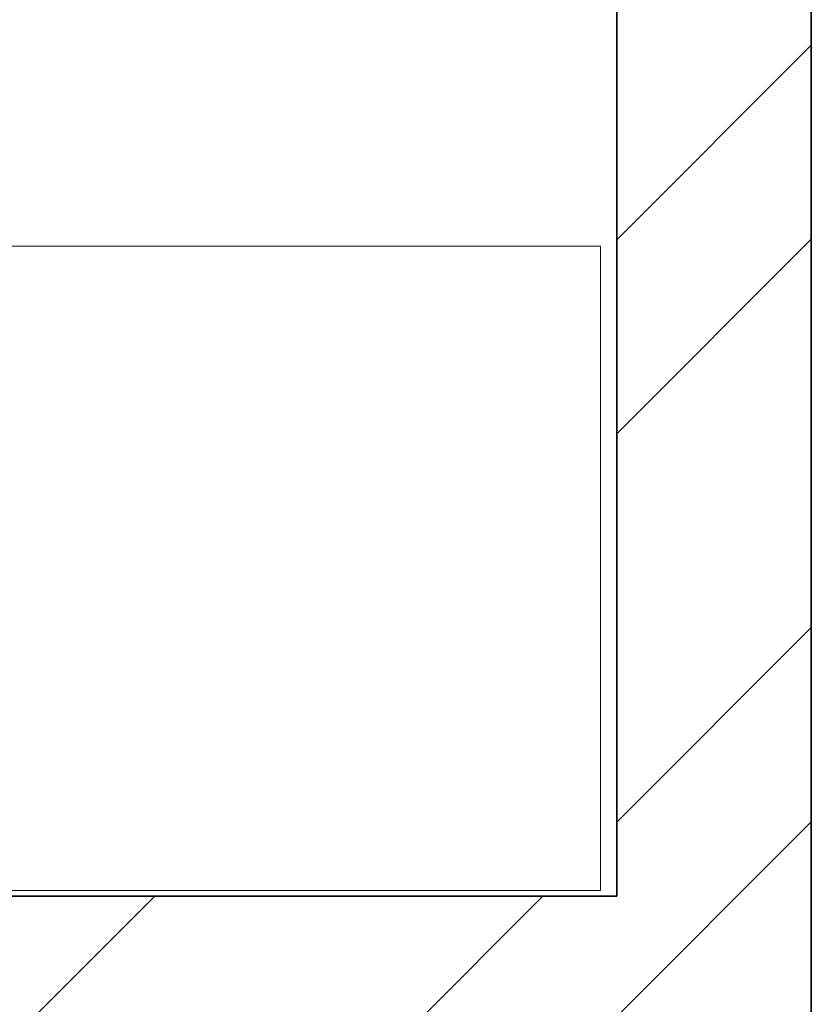
# Model space of a CAD drawing. Units: inches. Extents: x 2168 to 3056, y 1130 to 2629.
# Tile 40 of 42: x 2846 to 2864, y 2263 to 2286. Entities that reach past the tile are written whole.
import ezdxf

# ---------------------------------------------------------------- set-up
doc = ezdxf.new("R2010")
doc.units = ezdxf.units.IN
doc.layers.add('A-FLOR-CASE', color=71, linetype='Continuous', lineweight=18)
doc.layers.add('A-WALL', color=7, linetype='Continuous', lineweight=35)
doc.layers.add('A-WALL-PATT', color=143, linetype='Continuous', lineweight=13, true_color=0x7aafdf)

# ---------------------------------------------------------------- blocks, each defined once
blk = doc.blocks.new('CUPBOARD-BEDROOM')
blk.add_lwpolyline([(0, 14.894), (70.359, 14.894), (70.359, 0), (0, 0)], close=True)

msp = doc.modelspace()

# ---------------------------------------------------------------- hatches: boundary and pattern name
at = {"layer": 'A-WALL-PATT'}
h = msp.add_hatch(dxfattribs=at)
h.set_pattern_fill('ANSI32', color=256)
h.paths.add_polyline_path([(2463.796, 2409.389), (2467.387, 2409.389), (2467.387, 2413.889), (2454.768, 2413.889), (2454.768, 2411.639), (2454.768, 2409.389), (2459.296, 2409.389), (2459.296, 2265.389), (2455.644, 2265.389), (2455.644, 2260.889), (2467.349, 2260.889), (2467.349, 2263.139), (2467.349, 2265.389), (2463.796, 2265.389)])
h.paths.add_polyline_path([(2431.596, 2413.889), (2409.647, 2413.889), (2409.647, 2409.389), (2431.596, 2409.389), (2431.596, 2411.639)])
h.paths.add_polyline_path([(2349.647, 2413.889), (2331.796, 2413.889), (2331.796, 2362.671), (2336.296, 2362.671), (2336.296, 2409.389), (2349.647, 2409.389), (2349.647, 2411.639)])
h.paths.add_polyline_path([(2634.149, 2411.639), (2634.149, 2413.889), (2562.293, 2413.889), (2562.293, 2409.389), (2595.796, 2409.389), (2595.796, 2280.309), (2595.826, 2280.309), (2595.826, 2265.389), (2499.91, 2265.389), (2499.91, 2260.889), (2550.796, 2260.889), (2550.796, 2117.308), (2555.296, 2117.308), (2555.296, 2168.08), (2571.93, 2168.08), (2571.93, 2176.889), (2559.796, 2176.889), (2559.796, 2256.389), (2640.796, 2256.389), (2640.796, 2176.889), (2626.428, 2176.889), (2626.428, 2168.08), (2645.296, 2168.08), (2645.296, 2116.637), (2649.796, 2116.637), (2649.796, 2260.889), (2691.251, 2260.889), (2691.251, 2263.139), (2691.251, 2265.389), (2670.655, 2265.389), (2670.655, 2265.365), (2600.296, 2265.365), (2600.296, 2280.258), (2600.296, 2409.389), (2634.149, 2409.389)])
h.paths.add_polyline_path([(2600.296, 2473.889), (2612.84, 2473.889), (2612.84, 2478.389), (2572.636, 2478.389), (2572.636, 2473.889), (2595.796, 2473.889), (2595.796, 2413.889), (2600.296, 2413.889)])
h.paths.add_polyline_path([(2535.796, 2473.889), (2548.636, 2473.889), (2548.636, 2478.389), (2531.396, 2478.389), (2531.396, 2413.889), (2521.6, 2413.889), (2521.6, 2409.389), (2539.239, 2409.389), (2539.239, 2411.639), (2539.239, 2413.889), (2535.796, 2413.889)])
h.paths.add_polyline_path([(2664.796, 2478.389), (2636.84, 2478.389), (2636.84, 2473.889), (2660.296, 2473.889), (2660.296, 2413.889), (2656.165, 2413.889), (2656.165, 2409.389), (2671.684, 2409.389), (2671.684, 2411.639), (2671.684, 2413.889), (2664.796, 2413.889)])
h.paths.add_polyline_path([(2705.942, 2413.889), (2695.684, 2413.889), (2695.684, 2409.389), (2705.942, 2409.389)])
h.paths.add_polyline_path([(2741.35, 2413.889), (2728.733, 2413.889), (2728.733, 2411.639), (2728.733, 2409.389), (2732.296, 2409.389), (2732.296, 2265.389), (2725.733, 2265.389), (2725.733, 2260.889), (2740.917, 2260.889), (2740.917, 2263.139), (2740.917, 2265.389), (2736.796, 2265.389), (2736.796, 2409.389), (2741.35, 2409.389)])
h.paths.add_polyline_path([(2785.655, 2413.889), (2764.546, 2413.889), (2764.486, 2409.389), (2785.655, 2409.389), (2785.655, 2411.639)])
h.paths.add_polyline_path([(2864.296, 2413.889), (2845.655, 2413.889), (2845.655, 2409.389), (2859.796, 2409.389), (2859.796, 2368.425), (2864.296, 2368.425)])
h.paths.add_polyline_path([(2864.296, 2308.425), (2862.046, 2308.425), (2859.796, 2308.425), (2859.796, 2265.389), (2774.483, 2265.389), (2774.483, 2263.139), (2774.483, 2260.889), (2781.796, 2260.889), (2781.796, 2226.654), (2786.296, 2226.654), (2786.296, 2260.889), (2859.796, 2260.889), (2859.796, 2241.352), (2864.296, 2241.352)])
h.paths.add_polyline_path([(2864.296, 2217.352), (2862.046, 2217.352), (2859.796, 2217.352), (2859.796, 2200.889), (2786.296, 2200.889), (2786.296, 2205.931), (2784.046, 2205.931), (2781.796, 2205.931), (2781.796, 2150.974), (2786.296, 2150.974), (2786.296, 2161.889), (2859.796, 2161.889), (2859.796, 2144.419), (2864.296, 2144.419)])
h.paths.add_polyline_path([(2859.796, 2196.389), (2859.796, 2166.389), (2786.296, 2166.389), (2786.296, 2196.389)], flags=16)
h.paths.add_polyline_path([(2864.296, 2108.419), (2862.046, 2108.419), (2859.796, 2108.419), (2859.796, 2080.889), (2786.296, 2080.889), (2786.296, 2111.993), (2781.796, 2111.993), (2781.796, 2080.889), (2649.796, 2080.889), (2649.796, 2086.036), (2647.546, 2086.036), (2645.296, 2086.036), (2645.296, 2071.739), (2649.796, 2071.739), (2649.796, 2076.389), (2781.796, 2076.389), (2781.796, 2041.792), (2786.296, 2041.792), (2786.296, 2076.389), (2859.796, 2076.389), (2859.796, 2058.577), (2864.296, 2058.577)])
h.paths.add_polyline_path([(2864.296, 2022.577), (2859.796, 2022.577), (2859.796, 1992.389), (2786.296, 1992.389), (2786.296, 1999.573), (2781.796, 1999.573), (2781.796, 1848.085), (2784.046, 1848.085), (2786.296, 1848.085), (2786.296, 1851.389), (2859.796, 1851.389), (2859.796, 1838.258), (2864.296, 1838.258)], flags=17)
h.paths.add_polyline_path([(2859.796, 1987.889), (2859.796, 1855.889), (2786.296, 1855.889), (2786.296, 1987.889)], flags=16)
h.paths.add_polyline_path([(2823.046, 1987.889), (2841.421, 1921.889), (2823.046, 1855.889)], flags=0)
h.paths.add_polyline_path([(2864.296, 1814.258), (2859.796, 1814.258), (2859.796, 1791.389), (2786.296, 1791.389), (2786.296, 1825.658), (2784.046, 1825.658), (2781.796, 1825.658), (2781.796, 1791.389), (2720.155, 1791.389), (2720.155, 1791.265), (2649.796, 1791.265), (2649.796, 1806.159), (2649.796, 2038.983), (2647.546, 2038.983), (2645.296, 2038.983), (2645.296, 1783.925), (2649.796, 1783.925), (2649.796, 1786.889), (2781.796, 1786.889), (2781.796, 1746.789), (2786.296, 1746.789), (2786.296, 1786.889), (2859.796, 1786.889), (2859.796, 1770.083), (2864.296, 1770.083)])
h.paths.add_polyline_path([(2864.296, 1734.083), (2862.046, 1734.083), (2859.796, 1734.083), (2859.796, 1705.889), (2786.296, 1705.889), (2786.296, 1714.166), (2781.796, 1714.166), (2781.796, 1660.527), (2786.296, 1660.527), (2786.296, 1666.889), (2859.796, 1666.889), (2859.796, 1648.342), (2864.296, 1648.342)])
h.paths.add_polyline_path([(2786.296, 1701.389), (2859.796, 1701.389), (2859.796, 1671.389), (2786.296, 1671.389)], flags=16)
h.paths.add_polyline_path([(2649.796, 1756.576), (2647.546, 1756.576), (2645.296, 1756.576), (2645.296, 1606.889), (2555.296, 1606.889), (2555.296, 1749.513), (2553.046, 1749.513), (2550.796, 1749.513), (2550.796, 1606.889), (2503.006, 1606.889), (2503.006, 1604.639), (2503.006, 1602.389), (2595.796, 1602.389), (2595.849, 1602.389), (2595.849, 1587.495), (2595.796, 1458.389), (2561.502, 1458.389), (2561.502, 1456.139), (2561.502, 1453.889), (2595.796, 1453.889), (2595.796, 1381.889), (2573.438, 1381.889), (2573.438, 1377.389), (2613.01, 1377.389), (2613.01, 1379.639), (2613.01, 1381.889), (2600.296, 1381.889), (2600.296, 1453.889), (2634.327, 1453.889), (2634.327, 1458.389), (2600.296, 1458.389), (2600.296, 1602.389), (2670.655, 1602.389), (2694.095, 1602.389), (2694.095, 1606.889), (2649.796, 1606.889)])
h.paths.add_polyline_path([(2736.796, 1602.389), (2741.562, 1602.389), (2741.562, 1606.889), (2726.203, 1606.889), (2726.203, 1604.639), (2726.203, 1602.389), (2732.296, 1602.389), (2732.296, 1458.389), (2727.899, 1458.389), (2727.899, 1453.889), (2740.821, 1453.889), (2740.821, 1456.139), (2740.821, 1458.389), (2736.796, 1458.389)])
h.paths.add_polyline_path([(2859.796, 1606.889), (2786.296, 1606.889), (2786.296, 1637.334), (2784.046, 1637.334), (2781.796, 1637.334), (2781.796, 1606.889), (2775.612, 1606.889), (2775.612, 1602.389), (2859.796, 1602.389)])
h.paths.add_polyline_path([(2864.296, 1624.342), (2862.046, 1624.342), (2859.796, 1624.342), (2859.796, 1570.39), (2864.296, 1570.39)])
h.paths.add_polyline_path([(2864.296, 1510.39), (2862.046, 1510.39), (2859.796, 1510.39), (2859.796, 1458.389), (2846.735, 1458.389), (2846.735, 1456.139), (2846.735, 1453.889), (2864.296, 1453.889)])
h.paths.add_polyline_path([(2786.735, 1458.389), (2765.444, 1458.389), (2765.444, 1453.889), (2786.735, 1453.889)])
h.paths.add_polyline_path([(2706.004, 1458.389), (2695.36, 1458.389), (2695.36, 1453.889), (2706.004, 1453.889), (2706.004, 1456.139)])
h.paths.add_polyline_path([(2671.36, 1456.139), (2671.36, 1458.389), (2655.986, 1458.389), (2655.986, 1456.139), (2655.986, 1453.889), (2660.296, 1453.889), (2660.296, 1381.889), (2637.01, 1381.889), (2637.01, 1377.389), (2664.796, 1377.389), (2664.796, 1453.889), (2671.36, 1453.889)], flags=17)
h.paths.add_polyline_path([(2539.829, 1458.389), (2520.237, 1458.389), (2520.237, 1453.889), (2531.296, 1453.889), (2531.296, 1377.389), (2546.449, 1377.389), (2546.449, 1379.639), (2546.449, 1381.889), (2535.796, 1381.889), (2535.796, 1453.889), (2539.829, 1453.889)], flags=17)
h.paths.add_polyline_path([(2496.237, 1458.389), (2489.13, 1458.389), (2489.13, 1453.889), (2496.237, 1453.889), (2496.237, 1456.139)])
h.paths.add_polyline_path([(2467.433, 1456.139), (2467.433, 1458.389), (2463.796, 1458.389), (2463.796, 1602.389), (2468.242, 1602.389), (2468.242, 1605.7), (2468.242, 1606.889), (2454.602, 1606.889), (2454.602, 1602.389), (2459.296, 1602.389), (2459.296, 1458.389), (2454.24, 1458.389), (2454.24, 1453.889), (2467.433, 1453.889)])
h.paths.add_polyline_path([(2431.601, 1456.139), (2431.601, 1458.389), (2411.386, 1458.389), (2411.386, 1453.889), (2431.601, 1453.889)])
h.paths.add_polyline_path([(2351.386, 1458.389), (2336.296, 1458.389), (2336.296, 1490.693), (2334.046, 1490.693), (2331.796, 1490.693), (2331.796, 1453.889), (2351.386, 1453.889), (2351.386, 1456.139)])
h.paths.add_polyline_path([(2336.296, 1629.705), (2331.796, 1629.705), (2331.796, 1552.317), (2336.296, 1552.317), (2336.296, 1602.389), (2406.655, 1602.389), (2423.472, 1602.389), (2423.472, 1606.889), (2418.796, 1606.889), (2418.796, 1643.678), (2416.546, 1643.678), (2414.296, 1643.678), (2414.296, 1606.889), (2336.296, 1606.889)])
h.paths.add_polyline_path([(2418.796, 1714.384), (2414.296, 1714.384), (2414.296, 1705.889), (2336.296, 1705.889), (2336.296, 1731.324), (2334.046, 1731.324), (2331.796, 1731.324), (2331.796, 1653.705), (2334.046, 1653.705), (2336.296, 1653.705), (2336.296, 1666.889), (2414.296, 1666.889), (2414.296, 1663.589), (2418.796, 1663.589)])
h.paths.add_polyline_path([(2336.296, 1701.389), (2414.296, 1701.389), (2414.296, 1671.389), (2336.296, 1671.389)], flags=16)
h.paths.add_polyline_path([(2555.296, 2040.059), (2550.796, 2040.059), (2550.796, 1791.389), (2550.561, 1791.205), (2480.202, 1791.205), (2418.796, 1791.389), (2418.796, 1825.448), (2416.546, 1825.448), (2414.296, 1825.448), (2414.296, 1791.389), (2336.296, 1791.389), (2336.296, 1806.409), (2331.796, 1806.409), (2331.796, 1767.324), (2336.296, 1767.324), (2336.296, 1786.889), (2414.296, 1786.889), (2414.296, 1745.457), (2418.796, 1745.457), (2418.796, 1786.889), (2550.796, 1786.889), (2550.796, 1783.011), (2555.296, 1783.011)])
h.paths.add_polyline_path([(2418.796, 1923.389), (2423.207, 1923.389), (2423.207, 1925.639), (2423.207, 1927.889), (2418.796, 1927.889), (2418.796, 2000.048), (2414.296, 2000.048), (2414.296, 1992.389), (2336.296, 1992.389), (2336.296, 1987.889), (2414.296, 1987.889), (2414.296, 1855.889), (2336.296, 1855.889), (2336.296, 1851.389), (2414.296, 1851.389), (2414.296, 1846.759), (2418.796, 1846.759)], flags=17)
h.paths.add_polyline_path([(2336.296, 2019.294), (2334.046, 2019.294), (2331.796, 2019.294), (2331.796, 1830.409), (2336.296, 1830.409)], flags=17)
h.paths.add_polyline_path([(2550.796, 1927.889), (2453.541, 1927.889), (2453.541, 1925.639), (2453.541, 1923.389), (2550.796, 1923.389)], flags=17)
h.paths.add_polyline_path([(2744.987, 1927.889), (2649.796, 1927.889), (2649.796, 1923.389), (2744.987, 1923.389), (2744.987, 1925.639)], flags=17)
h.paths.add_polyline_path([(2555.296, 2086.458), (2553.046, 2086.458), (2550.796, 2086.458), (2550.796, 2080.889), (2418.796, 2080.889), (2336.296, 2080.889), (2336.296, 2115.399), (2334.046, 2115.399), (2331.796, 2115.399), (2331.796, 2055.294), (2336.296, 2055.294), (2336.296, 2076.389), (2550.796, 2076.389), (2550.796, 2071.538), (2555.296, 2071.538)])
h.paths.add_polyline_path([(2418.796, 2121.389), (2414.296, 2121.389), (2414.296, 2080.889), (2418.796, 2080.889)])
h.paths.add_polyline_path([(2418.796, 2076.389), (2414.296, 2076.389), (2414.296, 2035.123), (2418.796, 2035.123)])
h.paths.add_polyline_path([(2422.868, 2263.139), (2422.868, 2265.389), (2406.655, 2265.389), (2406.655, 2265.359), (2336.296, 2265.359), (2336.296, 2280.252), (2336.296, 2302.671), (2334.046, 2302.671), (2331.796, 2302.671), (2331.796, 2246.853), (2336.296, 2246.853), (2336.296, 2260.889), (2414.296, 2260.889), (2414.296, 2223.996), (2418.796, 2223.996), (2418.796, 2260.889), (2422.868, 2260.889)])
h.paths.add_polyline_path([(2418.796, 2204.783), (2416.546, 2204.783), (2414.296, 2204.783), (2414.296, 2200.889), (2336.296, 2200.889), (2336.296, 2220.853), (2331.796, 2220.853), (2331.796, 2151.399), (2336.296, 2151.399), (2336.296, 2161.889), (2414.296, 2161.889), (2414.296, 2153.726), (2418.796, 2153.726)])
h.paths.add_polyline_path([(2414.296, 2196.389), (2414.296, 2166.389), (2336.296, 2166.389), (2336.296, 2196.389)], flags=16)
h.paths.add_polyline_path([(2375.296, 2181.389), (2336.296, 2166.389), (2336.296, 2196.389)], flags=0)
h.paths.add_polyline_path([(2809.595, 2172.34), (2838.804, 2172.34), (2838.804, 2190.997), (2809.595, 2190.997)], flags=8)
h.paths.add_polyline_path([(2849.75, 1919.585), (2849.75, 1952.672), (2831.093, 1952.672), (2831.093, 1919.585)], flags=8)
h.paths.add_polyline_path([(2808.875, 1901.967), (2808.875, 1937.85), (2790.149, 1937.85), (2790.149, 1901.967)], flags=8)
h.paths.add_polyline_path([(2806.285, 1671.896), (2835.493, 1671.896), (2835.493, 1690.553), (2806.285, 1690.553)], flags=8)
h.paths.add_polyline_path([(2353.186, 1676.549), (2382.395, 1676.549), (2382.395, 1695.207), (2353.186, 1695.207)], flags=8)
h.paths.add_polyline_path([(2360.083, 1832.308), (2389.241, 1832.308), (2389.241, 1850.966), (2360.083, 1850.966)], flags=25)
h.paths.add_polyline_path([(2354.822, 2167.823), (2384.031, 2167.823), (2384.031, 2186.481), (2354.822, 2186.481)], flags=8)

# ---------------------------------------------------------------- linework, layer by layer
at = {"layer": 'A-WALL'}
for p, q in [((2859.796, 2308.425), (2859.796, 2265.389)), ((2864.296, 2308.425), (2864.296, 2241.352)), ((2772.841, 2265.389), (2859.796, 2265.389))]:
    msp.add_line(p, q, dxfattribs=at)

# ---------------------------------------------------------------- block references
at = {"layer": 'A-FLOR-CASE'}
msp.add_blockref('CUPBOARD-BEDROOM', (2789.057, 2265.523), dxfattribs=at)

doc.saveas('drawing.dxf')
